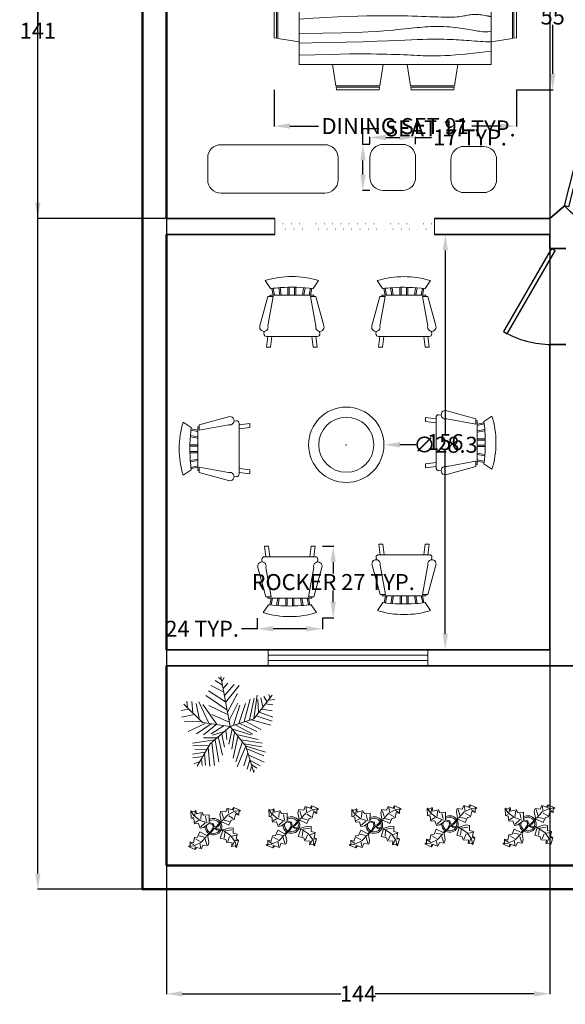
# Model space of a CAD drawing. Units: inches. Extents: x 823 to 1335, y 207 to 1074.
# Tile 1 of 6: x 823 to 1028, y 207 to 577. Entities that reach past the tile are written whole.
import ezdxf

# ---------------------------------------------------------------- set-up
doc = ezdxf.new("R2010")
doc.units = ezdxf.units.IN
doc.header["$MEASUREMENT"] = 0
doc.linetypes.add('ACAD_ISO07W100', pattern=[3, 0, -3])
for name, color, linetype, lineweight in [('A-ANNO-DIMS', 2, 'Continuous', 18), ('A-GLAZ-OVHD', 211, 'ACAD_ISO07W100', 18), ('doors', 51, 'Continuous', 25), ('furniture', 21, 'Continuous', 18), ('inner wall', 102, 'Continuous', 35), ('L-PLNT', 90, 'Continuous', 13), ('outer wall', 105, 'Continuous', 50), ('windows', 211, 'Continuous', 18)]:
    doc.layers.add(name, color=color, linetype=linetype, lineweight=lineweight)
doc.styles.get("Standard").update_dxf_attribs({"font": 'arial.ttf'})
doc.dimstyles.get("Standard").update_dxf_attribs({"dimtxt": 6, "dimasz": 6, "dimexe": 0.18, "dimexo": 0.0625, "dimgap": 0.09, "dimtad": 0, "dimtih": 1, "dimtoh": 1, "dimdec": 0, "dimzin": 0, "dimdsep": 46, "dimlunit": 3, "dimtxsty": 'Standard', "dimcen": 0.09, "dimadec": 0, "dimazin": 0, "dimtfac": 1, "dimtdec": 0, "dimtofl": 0, "dimtmove": 0, "dimatfit": 3, "dimfxl": 1, "dimtolj": 1, "dimtzin": 0, "dimarcsym": 0})

# ---------------------------------------------------------------- blocks, each defined once
blk = doc.blocks.new('*U5')
for p, q in [((0, 0), (0, -6)), ((-40, 0), (-40, -6))]:
    blk.add_line(p, q)
blk.add_lwpolyline([(0, 0), (-34.64, 20), (-35.52, 18.48), (-0.88, -1.52)], close=True)
blk.add_arc((0, 0), 40, 150, 180)
blk = doc.blocks.new('*U4')
for p, q in [((-40, 0), (-40, 6)), ((0, 0), (0, 6))]:
    blk.add_line(p, q)
blk.add_lwpolyline([(0, 0), (-34.64, -20), (-35.52, -18.48), (-0.88, 1.52)], close=True)
blk.add_arc((0, 0), 40, 180, 210)
blk = doc.blocks.new('Dining Set - 36 x 72 in.')
for p, q in [((-22.2343, 26.00059), (-23.4847, 17.99762)), ((-22.2304, 26), (-5.7608, 26)), ((-22, 27.5), (-22.1562, 26.50042)), ((-5.8416, 26.5), (-22.1534, 26.5)), ((-22, 27.5), (-6, 27.5)), ((-5.8437, 26.49966), (-6, 27.5)), ((-4.5152, 17.99762), (-5.7655, 25.99926)), ((5.7657, 26.00059), (4.5153, 17.99762)), ((5.7696, 26), (22.2392, 26)), ((6, 27.5), (5.8438, 26.50042)), ((22.1584, 26.5), (5.8466, 26.5)), ((6, 27.5), (22, 27.5)), ((22.1563, 26.49966), (22, 27.5)), ((23.4848, 17.99762), (22.2345, 25.99926)), ((36, 18), (-36, 18)), ((-36, 18), (-36, -18)), ((36, -18), (36, 18)), ((-45.5, 8), (-44.5004, 8.15617)), ((-45.5, 8), (-45.5, -8)), ((-44.5, -8.15843), (-44.5, 8.15338)), ((-44.0006, 8.23428), (-35.9976, 9.48474)), ((-44, 8.23041), (-44, -8.23915)), ((44.0006, 8.23428), (35.9976, 9.48474)), ((44, 8.23041), (44, -8.23915)), ((44.5, -8.15843), (44.5, 8.15338)), ((45.5, 8), (44.5005, 8.15617)), ((45.5, 8), (45.5, -8)), ((-44.4997, -8.15631), (-45.5, -8)), ((-35.9976, -9.48476), (-43.9993, -8.2345)), ((35.9976, -9.48476), (43.9993, -8.2345)), ((44.4997, -8.15631), (45.5, -8)), ((-36, -18), (36, -18)), ((-22.2343, -26.0006), (-23.4847, -17.99762)), ((-4.5152, -17.99762), (-5.7655, -25.99928)), ((5.7657, -26.0006), (4.5153, -17.99762)), ((23.4848, -17.99762), (22.2345, -25.99928)), ((-22.2304, -26), (-5.7608, -26)), ((-22, -27.5), (-22.1562, -26.50044)), ((-5.8416, -26.5), (-22.1534, -26.5)), ((-22, -27.5), (-6, -27.5)), ((-5.8437, -26.49967), (-6, -27.5)), ((5.7696, -26), (22.2392, -26)), ((6, -27.5), (5.8438, -26.50044)), ((22.1584, -26.5), (5.8466, -26.5)), ((6, -27.5), (22, -27.5)), ((22.1563, -26.49967), (22, -27.5))]:
    blk.add_line(p, q)
for points in [[(-36, 15), (-31.1772, 14.97754), (-26.8079, 14.91406), (-22.8538, 14.81543), (-19.276, 14.6875), (-16.0362, 14.53613), (-13.0957, 14.36718), (-10.4159, 14.18652), (-7.9583, 14), (-5.6904, 13.81315), (-3.6035, 13.63021), (-1.6954, 13.45508), (0.0365, 13.29166), (1.5945, 13.14388), (2.9811, 13.01562), (4.1988, 12.9108), (5.25, 12.83333), (6.1393, 12.78613), (6.8802, 12.76823), (7.4883, 12.77767), (7.9792, 12.8125), (8.3685, 12.87077), (8.6719, 12.95052), (8.9049, 13.0498), (9.0833, 13.16666), (9.2205, 13.29899), (9.3216, 13.44401), (9.3895, 13.59879), (9.4271, 13.76041), (9.4373, 13.92594), (9.4232, 14.09245), (9.3875, 14.257), (9.3333, 14.41666), (9.2638, 14.56917), (9.1836, 14.71484), (9.0975, 14.85465), (9.0104, 14.98958), (8.9272, 15.1206), (8.8529, 15.2487), (8.7922, 15.37483), (8.75, 15.5), (8.7305, 15.62467), (8.7344, 15.74739), (8.7617, 15.86621), (8.8125, 15.97916), (8.8867, 16.08431), (8.9844, 16.17968), (9.1055, 16.26334), (9.25, 16.33333), (9.4189, 16.38802), (9.6172, 16.42708), (9.8506, 16.45052), (10.125, 16.45833), (10.4463, 16.45052), (10.8203, 16.42708), (11.2529, 16.38802), (11.75, 16.33333), (12.3184, 16.26318), (12.9694, 16.17838), (13.7151, 16.07991), (14.5677, 15.96875), (15.5395, 15.84586), (16.6426, 15.71224), (17.8893, 15.56884), (19.2917, 15.41666), (20.859, 15.25667), (22.5879, 15.08984), (24.4721, 14.91715), (26.5052, 14.73958), (28.6809, 14.5581), (30.9929, 14.3737), (33.4347, 14.18733), (36, 14)], [(-36, 10), (-28.9766, 10.14274), (-23.1725, 10.20442), (-18.4241, 10.19775), (-14.5677, 10.13541), (-11.4399, 10.03011), (-8.877, 9.89453), (-6.7154, 9.74137), (-4.7917, 9.58333), (-2.9698, 9.43082), (-1.2246, 9.28515), (0.4415, 9.14534), (2.026, 9.01041), (3.5266, 8.87939), (4.9408, 8.7513), (6.266, 8.62516), (7.5, 8.5), (8.6411, 8.37549), (9.6914, 8.2539), (10.6538, 8.13818), (11.5312, 8.03125), (12.3267, 7.93603), (13.043, 7.85547), (13.6831, 7.79248), (14.25, 7.75), (14.7471, 7.7303), (15.1797, 7.73307), (15.5537, 7.75732), (15.875, 7.80208), (16.1494, 7.86637), (16.3828, 7.94922), (16.5811, 8.04964), (16.75, 8.16666), (16.8944, 8.29915), (17.0143, 8.44531), (17.1089, 8.60319), (17.1771, 8.77083), (17.218, 8.94629), (17.2305, 9.1276), (17.2137, 9.31282), (17.1667, 9.5), (17.0895, 9.6875), (16.987, 9.875), (16.8649, 10.0625), (16.7292, 10.25), (16.5856, 10.4375), (16.4401, 10.625), (16.2985, 10.8125), (16.1667, 11), (16.05, 11.18733), (15.9518, 11.3737), (15.8752, 11.5581), (15.8229, 11.73958), (15.798, 11.91715), (15.8034, 12.08984), (15.842, 12.25667), (15.9167, 12.41666), (16.0295, 12.56836), (16.1784, 12.70833), (16.3605, 12.83268), (16.5729, 12.9375), (16.8127, 13.01888), (17.0768, 13.07291), (17.3625, 13.0957), (17.6667, 13.08333), (17.9894, 13.03312), (18.3418, 12.94726), (18.7382, 12.82918), (19.1927, 12.68229), (19.7195, 12.51001), (20.3327, 12.31575), (21.0465, 12.10294), (21.875, 11.875), (22.8357, 11.63354), (23.959, 11.37304), (25.2786, 11.08618), (26.8282, 10.76562), (28.6414, 10.40405), (30.752, 9.99414), (33.1936, 9.52856), (36, 9)], [(-36, 5.5), (-30.7157, 5.3348), (-26.069, 5.20963), (-21.9946, 5.11767), (-18.4271, 5.05208), (-15.3009, 5.00602), (-12.5508, 4.97265), (-10.1112, 4.94515), (-7.9167, 4.91666), (-5.909, 4.88167), (-4.0586, 4.83984), (-2.3429, 4.79215), (-0.7396, 4.73958), (0.7739, 4.6831), (2.22, 4.6237), (3.6213, 4.56233), (5, 4.5), (6.373, 4.43782), (7.7344, 4.3776), (9.0723, 4.32129), (10.375, 4.27083), (11.6309, 4.22819), (12.8281, 4.19531), (13.9551, 4.17415), (15, 4.16666), (15.954, 4.17448), (16.819, 4.19791), (17.6001, 4.23698), (18.3021, 4.29166), (18.9299, 4.36198), (19.4883, 4.44791), (19.9823, 4.54948), (20.4167, 4.66666), (20.7969, 4.79899), (21.1302, 4.94401), (21.4245, 5.09879), (21.6875, 5.26041), (21.9271, 5.42594), (22.1511, 5.59245), (22.3672, 5.757), (22.5834, 5.91666), (22.8065, 6.06868), (23.0404, 6.21093), (23.2879, 6.34147), (23.5521, 6.45833), (23.8358, 6.55957), (24.142, 6.64323), (24.4735, 6.70735), (24.8334, 6.75), (25.2235, 6.76969), (25.642, 6.76692), (26.0858, 6.74267), (26.5521, 6.69791), (27.0379, 6.63362), (27.5404, 6.55078), (28.0565, 6.45036), (28.5834, 6.33333), (29.1242, 6.19987), (29.7071, 6.04687), (30.3661, 5.87044), (31.1354, 5.66666), (32.0493, 5.43164), (33.142, 5.16146), (34.4475, 4.85221), (36, 4.5)], [(-36, -1), (-30.7915, -0.6591), (-26.0195, -0.38216), (-21.6519, -0.16284), (-17.6563, 0.00521), (-14.0005, 0.12833), (-10.6523, 0.21289), (-7.5796, 0.26522), (-4.75, 0.29166), (-2.134, 0.29793), (0.2878, 0.28711), (2.5317, 0.26163), (4.6146, 0.22396), (6.5529, 0.17651), (8.3633, 0.12174), (10.0623, 0.06209), (11.6667, 0), (13.1899, -0.06201), (14.6341, -0.1211), (15.9982, -0.17432), (17.2813, -0.21875), (18.4823, -0.25147), (19.6003, -0.26953), (20.6343, -0.27002), (21.5834, -0.25), (22.4481, -0.20768), (23.2357, -0.14584), (23.9549, -0.06836), (24.6146, 0.02083), (25.2235, 0.11784), (25.7904, 0.21875), (26.3241, 0.31966), (26.8334, 0.41666), (27.3265, 0.50618), (27.8099, 0.58593), (28.2894, 0.65397), (28.7709, 0.70833), (29.2601, 0.74707), (29.763, 0.76823), (30.2855, 0.76985), (30.8334, 0.75), (31.4088, 0.70784), (31.9994, 0.64713), (32.589, 0.57275), (33.1615, 0.48958), (33.7008, 0.4025), (34.1908, 0.3164), (34.6153, 0.23616), (34.9584, 0.16666), (35.2099, 0.11165), (35.3848, 0.07031), (35.504, 0.04069), (35.5886, 0.02083), (35.6594, 0.00879), (35.7377, 0.0026), (35.8442, 0.00032), (36, 0)], [(-36, -6.5), (-27.1843, -6.31267), (-20.084, -6.1263), (-14.469, -5.9419), (-10.1094, -5.76042), (-6.7752, -5.58285), (-4.2363, -5.41016), (-2.2629, -5.24333), (-0.625, -5.08334), (0.8708, -4.93099), (2.2715, -4.78646), (3.5872, -4.64974), (4.8281, -4.52084), (6.0046, -4.39974), (7.127, -4.28646), (8.2053, -4.18099), (9.25, -4.08334), (10.2705, -3.99382), (11.2734, -3.91407), (12.2647, -3.84603), (13.25, -3.79167), (14.2354, -3.75293), (15.2266, -3.73177), (16.2295, -3.73015), (17.25, -3.75), (18.2912, -3.79248), (19.3451, -3.85547), (20.4009, -3.93604), (21.4479, -4.03125), (22.4754, -4.13819), (23.4727, -4.25391), (24.4289, -4.37549), (25.3334, -4.5), (26.1785, -4.62492), (26.9694, -4.74935), (27.7145, -4.87281), (28.4219, -4.99479), (29.1, -5.11483), (29.7572, -5.23242), (30.4016, -5.34709), (31.0417, -5.45834), (31.6837, -5.56437), (32.3262, -5.65821), (32.9658, -5.73153), (33.599, -5.77604), (34.2224, -5.78345), (34.8327, -5.74545), (35.4264, -5.65373), (36, -5.5)], [(-36, -10), (-26.4022, -9.81299), (-18.4675, -9.62891), (-11.9839, -9.45069), (-6.7396, -9.28125), (-2.5226, -9.12354), (0.8789, -8.98047), (3.6769, -8.85498), (6.0833, -8.75), (8.2767, -8.66765), (10.3021, -8.60677), (12.1712, -8.56543), (13.8958, -8.54167), (15.4876, -8.53353), (16.9583, -8.53907), (18.3197, -8.55632), (19.5834, -8.58334), (20.7616, -8.61841), (21.8685, -8.66081), (22.9188, -8.71004), (23.9271, -8.76563), (24.9081, -8.82707), (25.8763, -8.89388), (26.8465, -8.96558), (27.8334, -9.04167), (28.8474, -9.12118), (29.8828, -9.20117), (30.93, -9.27824), (31.9792, -9.34896), (33.0205, -9.40991), (34.0443, -9.45768), (35.0407, -9.48885), (36, -9.5)], [(-36, -14.5), (-30.0881, -14.33513), (-25.0332, -14.21224), (-20.7312, -14.12647), (-17.0781, -14.07292), (-13.97, -14.04671), (-11.3027, -14.04297), (-8.9724, -14.05681), (-6.875, -14.08334), (-4.9224, -14.11833), (-3.0905, -14.16016), (-1.3709, -14.20785), (0.2448, -14.26042), (1.7647, -14.3169), (3.1973, -14.3763), (4.5507, -14.43767), (5.8333, -14.5), (7.0554, -14.5621), (8.235, -14.62175), (9.3922, -14.67652), (10.5469, -14.72396), (11.7192, -14.76164), (12.929, -14.78711), (14.1965, -14.79794), (15.5417, -14.79167), (16.9933, -14.76424), (18.6152, -14.70508), (20.4804, -14.60197), (22.6615, -14.44271), (25.2312, -14.21509), (28.2624, -13.9069), (31.8277, -13.50594), (36, -13)]]:
    blk.add_lwpolyline(points)
blk = doc.blocks.new('Chair - Rocking')
for p, q in [((-8, -4.5), (-10, -1.5)), ((8, -4.5), (10, -1.5)), ((-8.23428, -6.99939), (-8.3093, -7.47958)), ((-8.23041, -7), (8.23915, -7)), ((-7.5, -4.5), (-7, -7)), ((-6.5, -7), (-7.02225, -4.43)), ((-4.5, -7), (-4.96674, -4.19951)), ((-4, -7), (-4.40532, -4.16272)), ((-1.5, -4.05012), (-1.5, -7)), ((-1, -7), (-1, -4.05012)), ((1, -7), (1, -4.04655)), ((1.5, -4.05012), (1.5, -7)), ((4, -7), (4.40187, -4.18694)), ((4.5, -7), (4.96761, -4.19437)), ((6.5, -7), (7, -4.4057)), ((7.5, -4.5), (7, -7)), ((8.31071, -7.48854), (8.23449, -7.00073)), ((-9, -7.5), (-12, -18.49999)), ((-7, -7.5), (-9, -7.5)), ((-9, -18.49999), (-7, -7.5)), ((7, -7.5), (9, -7.5)), ((9, -18.49999), (7, -7.5)), ((9, -7.5), (12, -18.49999)), ((-10.36644, -20.64523), (-10.5, -21.49999)), ((10.5, -21.49999), (10.3575, -20.58798)), ((-9, -22.49999), (-9.5, -26.49999)), ((0, -22.49999), (-9.5, -22.49999)), ((-8, -26.49999), (-7.5, -22.49999)), ((0, -22.49999), (9.5, -22.49999)), ((8, -26.49999), (7.5, -22.49999)), ((9, -22.49999), (9.5, -26.49999)), ((-9.5, -26.49999), (-8, -26.49999)), ((9.5, -26.49999), (8, -26.49999))]:
    blk.add_line(p, q)
for centre, radius, start, end in [((0, -34.08333), 34.08333, 72.93847, 107.0615), ((0, -68.25004), 64.25, 93.92211, 97.15267), ((0, -68.25004), 64.25, 82.84733, 93.92211), ((-10.5, -18.99999), 1.58114, 161.5651, 18.43495), ((-9.5, -21.49999), 1, 180, 270), ((10.5, -18.99999), 1.58114, 161.5651, 18.43495), ((9.5, -21.49999), 1, 270, 0)]:
    blk.add_arc(centre, radius, start, end)
blk = doc.blocks.new('Plant - Rubber or Philodendron')
for p, q in [((-16.2005, 11.4774), (-13.9899, 8.1064)), ((-16.2005, 11.4774), (-14.8639, 10.7964)), ((-16.0159, 6.3329), (-16.2005, 11.4774)), ((-14.8639, 10.7964), (-12.6195, 11.8975)), ((-13.9899, 8.1064), (-9.5434, 4.7185)), ((-13.3174, 8.325), (-13.0735, 11.0065)), ((-12.6195, 11.8975), (-12.1909, 9.4345)), ((-12.1909, 9.4345), (-8.3829, 10.3)), ((-8.8369, 9.409), (-9.0894, 5.6095)), ((-8.3829, 10.3), (-7.0549, 8.501)), ((-7.0549, 8.501), (-3.0284, 8.6941)), ((-4.8529, 4.012), (-5.7184, 7.82)), ((-3.0284, 8.6941), (-3.0709, 3.1041)), ((4.6914, 8.8812), (5.3859, 11.2828)), ((4.6914, 8.8812), (5.5014, 4.4831)), ((5.3859, 11.2828), (8.8871, 10.7908)), ((5.9878, 10.4842), (7.1971, 6.3869)), ((10.3916, 8.7942), (6.2847, 4.4028)), ((8.8871, 10.7908), (9.9809, 13.4933)), ((9.9809, 13.4933), (13.3837, 12.301)), ((15.3859, 11.3055), (10.3916, 8.7942)), ((10.5828, 12.6946), (10.8893, 9.7953)), ((14.2977, 6.1031), (10.9934, 7.9956)), ((13.3837, 12.301), (14.68, 13.9039)), ((14.5816, 13.2037), (14.3848, 11.8033)), ((14.68, 13.9039), (19.3848, 11.8146)), ((15.7909, 9.1065), (14.8995, 5.3044)), ((15.2875, 10.6053), (17.5907, 9.2105)), ((19.3848, 11.8146), (15.3859, 11.3055)), ((18.1925, 8.4119), (15.7909, 9.1065)), ((19.3848, 11.8146), (18.1868, 10.9119)), ((18.1868, 10.9119), (18.1925, 8.4119)), ((-14.0069, 5.8704), (-16.0159, 6.3329)), ((-15.3434, 6.5514), (-13.9984, 6.9884)), ((-13.5868, 2.2894), (-14.0069, 5.8704)), ((-10.6784, 2.491), (-13.5868, 2.2894)), ((-13.1329, 3.1804), (-10.6614, 4.727)), ((-9.5858, -0.8715), (-10.6784, 2.491)), ((-9.5434, 4.7185), (-4.1917, 2.9888)), ((-9.1318, 0.0195), (-5.9793, 2.9025)), ((-7.1228, -0.443), (-3.5248, 2.2131)), ((-3.5248, 2.2131), (-3.3011, 2.4355)), ((-3.3011, 2.4355), (-0.5306, 1.7947)), ((-3.0709, 3.1041), (0.0797, 2.3163)), ((-0.5306, 1.7947), (-0.2255, -0.5527)), ((-0.5306, 1.7947), (-0.5306, 1.7947)), ((0.0797, 2.3163), (0.4866, -0.031)), ((0.4866, -0.031), (2.1141, 0.2298)), ((2.1141, 0.2298), (5.4346, 3.9146)), ((6.1032, 3.6844), (2.8262, -0.031)), ((5.4346, 3.9146), (5.5014, 4.4831)), ((11.1089, 1.1958), (6.1032, 3.6844)), ((7.7005, 4.8881), (11.5025, 3.9967)), ((12.7005, 4.8994), (11.1089, 1.1958)), ((14.8995, 5.3044), (12.7005, 4.8994)), ((-11.3237, -7.2629), (-9.7321, -3.5593)), ((-6.3237, -7.2516), (-10.1257, -6.3602)), ((-9.7321, -3.5593), (-4.7264, -6.0479)), ((-7.1228, -0.443), (-9.5858, -0.8715)), ((-9.0148, -11.1577), (-4.9047, -6.8122)), ((-2.019, -3.6148), (-4.7264, -6.0479)), ((-4.1246, -6.8466), (-4.0579, -6.2781)), ((-3.3146, -11.2447), (-4.1246, -6.8466)), ((-4.0579, -6.2781), (-0.9375, -3.1608)), ((-2.019, -3.6148), (-0.2255, -0.5527)), ((-0.9375, -3.1608), (0.5883, -0.8135)), ((0.5883, -0.8135), (2.2447, -2.0916)), ((2.8262, -0.031), (1.3003, -0.5527)), ((1.3003, -0.5527), (2.4193, -1.4655)), ((2.2447, -2.0916), (6.7108, -2.6626)), ((2.4193, -1.4655), (6.895, -2.1175)), ((4.943, -7.9659), (6.7108, -2.6626)), ((11.6605, -0.5413), (6.895, -2.1175)), ((12.3677, -6.1981), (7.219, -2.6772)), ((8.125, -4.0768), (7.7715, -7.9659)), ((8.3544, -2.7453), (13.1973, -2.1704)), ((10.2463, -10.4408), (11.6605, -6.9053)), ((11.6605, -0.5413), (14.1354, -0.8948)), ((15.5496, -10.7943), (12.3677, -6.1981)), ((16.2567, -5.8446), (13.4283, -6.5517)), ((14.1354, -0.8948), (14.1354, -4.4304)), ((14.1354, -4.4304), (16.9638, -5.1375)), ((16.9638, -5.1375), (16.2567, -8.673)), ((-18.008, -14.1781), (-16.8101, -13.2754)), ((-18.008, -14.1781), (-14.0091, -13.669)), ((-16.8157, -10.7754), (-14.4141, -11.4699)), ((-16.8101, -13.2754), (-16.8157, -10.7754)), ((-13.9107, -12.9688), (-16.2139, -11.574)), ((-14.4141, -11.4699), (-13.5228, -7.6679)), ((-14.0091, -13.669), (-9.0148, -11.1577)), ((-13.5228, -7.6679), (-11.3237, -7.2629)), ((-12.921, -8.4665), (-9.6166, -10.359)), ((-9.206, -15.0581), (-9.5126, -12.1588)), ((-7.5103, -13.1543), (-8.6042, -15.8568)), ((-4.0092, -13.6463), (-7.5103, -13.1543)), ((-4.611, -12.8477), (-5.8203, -8.7504)), ((-3.3146, -11.2447), (-4.0092, -13.6463)), ((8.8321, -9.0266), (4.943, -7.9659)), ((9.5392, -11.1479), (8.8321, -9.0266)), ((13.4283, -11.5015), (9.5392, -11.1479)), ((13.0748, -13.9763), (13.4283, -11.5015)), ((15.5496, -13.6228), (13.0748, -13.9763)), ((14.8425, -10.7943), (13.7819, -13.2692)), ((16.6103, -14.6834), (15.5496, -10.7943)), ((16.6103, -14.6834), (15.5496, -13.6228)), ((17.3174, -9.7337), (15.9032, -9.7337)), ((16.2567, -8.673), (18.0245, -9.7337)), ((18.0245, -9.7337), (16.6103, -14.6834)), ((-13.3032, -16.2674), (-18.008, -14.1781)), ((-12.0069, -14.6645), (-13.3032, -16.2674)), ((-13.2048, -15.5672), (-13.008, -14.1668)), ((-8.6042, -15.8568), (-12.0069, -14.6645))]:
    blk.add_line(p, q)
for centre, radius, start, end in [((0.0308, 0.1664), 6, 178.6147, 235.1169), ((0.0308, 0.1664), 5, 168.1647, 238.6725), ((0, 0), 6.1275, 34.37569, 120.1028), ((-0.0601, -0.2075), 5.2461, 33.82192, 124.9414), ((-0.2664, 0.1682), 5.2775, 338.4094, 20.03007), ((-0.098, 0.1364), 6.1288, 341.2017, 26.09184), ((-0.0234, 0.3825), 6.1492, 242.5812, 331.2714), ((-0.1102, 0.4886), 5.2883, 247.3711, 327.472)]:
    blk.add_arc(centre, radius, start, end)
blk = doc.blocks.new('*U20')
for p, q in [((0, 0), (-10.5, 57)), ((-7.288, 39.707), (-21.778, 46.673)), ((-8.737, 47.138), (-17.069, 52.711)), ((-10.186, 53.64), (-13.084, 55.962)), ((-9.099, 51.782), (-6.563, 55.962)), ((-7.65, 43.423), (-2.578, 49.46)), ((-5.839, 35.992), (4.667, 48.067)), ((-5.114, 27.632), (10.463, 46.673)), ((-3.665, 19.273), (-27.574, 35.527)), ((-5.114, 28.097), (-24.676, 40.636)), ((-2.941, 16.486), (8.652, 37.85)), ((27, 9), (48, 36)), ((27.127, 9.056), (31.112, 35.992)), ((38.719, 34.134), (41.979, 28.561)), ((44.153, 36.456), (45.239, 32.741)), ((-31.5, 4.5), (-52.5, 25.5)), ((-48.585, 21.131), (-49.309, 29.026)), ((-43.513, 28.561), (-42.427, 15.558)), ((-38.442, 26.239), (-34.819, 7.663)), ((-35.544, 28.097), (-24.314, 3.947)), ((-14.533, 2.09), (-30.834, 25.31)), ((-24.314, 23.917), (-2.941, 13.7)), ((-1.129, 6.734), (9.014, 26.704)), ((3.942, 1.625), (11.187, 24.381)), ((10.101, 3.483), (17.708, 26.239)), ((16.259, 5.805), (23.142, 31.348)), ((22.055, 7.198), (27.489, 32.277)), ((31.836, 30.883), (32.561, 16.486)), ((35.096, 32.741), (37.27, 22.524)), ((40.53, 25.775), (48.862, 24.846)), ((43.791, 29.954), (51.036, 30.883)), ((-47.498, 19.737), (-55.83, 18.344)), ((-40.615, 13.7), (-55.105, 10.913)), ((-20.691, 13.7), (-1.129, 4.876)), ((29.662, 12.307), (48.137, 6.269)), ((33.285, 16.486), (48.862, 10.913)), ((36.183, 19.737), (48.137, 17.88)), ((-33.37, 6.269), (-52.207, 5.34)), ((-28.299, 3.483), (-47.86, -5.805)), ((-21.416, 3.018), (-38.079, -8.128)), ((0, 0), (-31.5, 4.5)), ((-15.982, 2.09), (-30.11, -9.521)), ((0, 0), (-22.5, -19.5)), ((-6.563, 1.161), (-21.416, -8.128)), ((0, 0), (27, 9)), ((0, 0), (18, -22.5)), ((6.478, 1.625), (26.04, -8.592)), ((11.187, 3.483), (30.749, -5.805)), ((18.07, 5.805), (35.096, -3.483)), ((24.229, 7.663), (46.688, 1.625)), ((-6.563, -5.805), (-19.967, -9.985)), ((-9.461, -8.592), (-6.201, -23.453)), ((-4.752, -3.483), (-3.665, -14.629)), ((2.493, -3.019), (-1.491, -20.202)), ((1.769, -2.555), (24.229, -9.521)), ((5.029, -6.27), (2.131, -25.775)), ((7.565, -9.056), (32.198, -14.629)), ((-17.431, -15.094), (-42.789, -18.809)), ((-24.314, -21.596), (-42.427, -22.06)), ((-22.5, -19.5), (-37.5, -45)), ((-15.257, -12.772), (-30.11, -12.772)), ((-20.691, -18.345), (-17.793, -44.352)), ((-17.069, -15.094), (-12.721, -40.172)), ((-13.446, -11.378), (-8.737, -32.741)), ((9.014, -11.378), (3.58, -35.992)), ((14.085, -16.951), (6.478, -40.172)), ((12.274, -15.094), (36.907, -18.809)), ((16.259, -19.738), (36.183, -22.989)), ((-28.299, -29.026), (-42.789, -31.348)), ((-26.849, -26.24), (-40.253, -25.775)), ((-29.023, -30.884), (-27.936, -43.887)), ((-25.038, -23.918), (-22.865, -45.281)), ((18.07, -22.524), (8.289, -45.745)), ((20.244, -30.419), (15.897, -44.816)), ((18, -22.5), (27, -52.5)), ((18.433, -22.524), (40.53, -29.026)), ((19.157, -25.311), (38.719, -33.206)), ((21.331, -32.741), (39.081, -40.636)), ((-30.834, -34.135), (-42.427, -35.528)), ((-34.457, -39.708), (-40.978, -42.494)), ((-32.646, -36.921), (-31.921, -44.352)), ((22.78, -37.85), (19.519, -48.532)), ((22.78, -38.314), (34.372, -44.816)), ((24.591, -43.423), (30.749, -47.603)), ((24.591, -45.745), (23.142, -50.854)), ((26.764, -49.925), (28.213, -50.854))]:
    blk.add_line(p, q)
blk = doc.blocks.new('WIN-60IN')
for p, q in [((0, 0), (0, 60)), ((0, 60), (6, 60)), ((2, 0), (2, 60)), ((4, 60), (4, 0)), ((6, 60), (6, 0)), ((6, 0), (0, 0))]:
    blk.add_line(p, q)
blk = doc.blocks.new('SEAT-HALL-SINGLE')
for points in [[(5, 17.36), (12.18, 17.36)], [(0, 5), (0, 12.36)], [(17.18, 12.36), (17.18, 5)], [(12.18, 0), (5, 0)]]:
    blk.add_lwpolyline(points)
for centre, start, end in [((5, 12.36), 90, 180), ((12.18, 12.36), 0, 90), ((5, 5), 180, 270), ((12.18, 5), 270, 0)]:
    blk.add_arc(centre, 5, start, end)
blk = doc.blocks.new('*D30')
at = {"layer": 'A-ANNO-DIMS', "color": 0, "lineweight": -2, "transparency": 16777216}
for p, q in [((918.69, 550.91), (918.69, 537.15)), ((1009.69, 550.91), (1009.69, 537.15)), ((924.69, 537.33), (935.39, 537.33)), ((1003.69, 537.33), (993, 537.33))]:
    blk.add_line(p, q, dxfattribs=at)
for points in [[(924.69, 538.33), (924.69, 536.33), (918.69, 537.33)], [(1003.69, 538.33), (1003.69, 536.33), (1009.69, 537.33)]]:
    blk.add_solid(points, dxfattribs=at)
at = {"layer": 'Defpoints', "color": 0, "lineweight": -2, "transparency": 16777216}
for p in [(918.69, 550.98), (1009.69, 550.98), (1009.69, 537.33)]:
    blk.add_point(p, dxfattribs=at)
at = {"layer": 'A-ANNO-DIMS', "color": 0, "transparency": 16777216, "insert": (964.19, 537.33), "char_height": 6, "attachment_point": 5}
blk.add_mtext('\\A1;DINING SET 91', dxfattribs=at)
blk = doc.blocks.new('*D31')
at = {"layer": 'A-ANNO-DIMS', "color": 0, "lineweight": -2, "transparency": 16777216}
for p, q in [((1009.76, 605.98), (1023.52, 605.98)), ((1023.34, 599.98), (1023.34, 581.62)), ((1023.34, 556.98), (1023.34, 575.34)), ((1009.76, 550.98), (1023.52, 550.98))]:
    blk.add_line(p, q, dxfattribs=at)
for points in [[(1022.34, 599.98), (1024.34, 599.98), (1023.34, 605.98)], [(1022.34, 556.98), (1024.34, 556.98), (1023.34, 550.98)]]:
    blk.add_solid(points, dxfattribs=at)
at = {"layer": 'Defpoints', "color": 0, "lineweight": -2, "transparency": 16777216}
for p in [(1009.69, 605.98), (1023.34, 605.98), (1009.69, 550.98)]:
    blk.add_point(p, dxfattribs=at)
at = {"layer": 'A-ANNO-DIMS', "color": 0, "transparency": 16777216, "insert": (1023.34, 578.48), "char_height": 6, "attachment_point": 5}
blk.add_mtext('\\A1;55', dxfattribs=at)
blk = doc.blocks.new('*D34')
at = {"layer": 'A-ANNO-DIMS', "color": 0, "lineweight": -2, "transparency": 16777216}
for p, q in [((936.93, 379.54), (941.1, 379.54)), ((940.92, 373.54), (940.92, 369.24)), ((940.92, 358.54), (940.92, 362.85)), ((936.93, 352.54), (941.1, 352.54))]:
    blk.add_line(p, q, dxfattribs=at)
for points in [[(939.92, 373.54), (941.92, 373.54), (940.92, 379.54)], [(939.92, 358.54), (941.92, 358.54), (940.92, 352.54)]]:
    blk.add_solid(points, dxfattribs=at)
at = {"layer": 'Defpoints', "color": 0, "lineweight": -2, "transparency": 16777216}
for p in [(936.87, 379.54), (936.87, 352.54), (940.92, 352.54)]:
    blk.add_point(p, dxfattribs=at)
at = {"layer": 'A-ANNO-DIMS', "color": 0, "transparency": 16777216, "insert": (940.92, 366.04), "char_height": 6, "attachment_point": 5}
blk.add_mtext('\\A1;ROCKER 27 TYP.', dxfattribs=at)
blk = doc.blocks.new('*D35')
at = {"layer": 'A-ANNO-DIMS', "color": 0, "lineweight": -2, "transparency": 16777216}
for p, q in [((912.43, 352.48), (912.43, 348.31)), ((936.87, 352.48), (936.87, 348.31)), ((912.43, 348.49), (906.43, 348.49)), ((930.87, 348.49), (918.43, 348.49))]:
    blk.add_line(p, q, dxfattribs=at)
for points in [[(918.43, 349.49), (918.43, 347.49), (912.43, 348.49)], [(930.87, 349.49), (930.87, 347.49), (936.87, 348.49)]]:
    blk.add_solid(points, dxfattribs=at)
at = {"layer": 'Defpoints', "color": 0, "lineweight": -2, "transparency": 16777216}
for p in [(912.43, 352.54), (936.87, 352.54), (912.43, 348.49)]:
    blk.add_point(p, dxfattribs=at)
at = {"layer": 'A-ANNO-DIMS', "color": 0, "transparency": 16777216, "insert": (891.69, 348.49), "char_height": 6, "attachment_point": 5}
blk.add_mtext('\\A1;24 TYP.', dxfattribs=at)
blk = doc.blocks.new('*D38')
at = {"layer": 'A-ANNO-DIMS', "color": 0, "lineweight": -2, "transparency": 16777216}
for p, q in [((952.1, 530.45), (952.1, 536.45)), ((952.1, 536.45), (958.1, 536.45)), ((954.64, 530.45), (951.92, 530.45)), ((952.1, 519.09), (952.1, 524.45)), ((954.64, 513.09), (951.92, 513.09))]:
    blk.add_line(p, q, dxfattribs=at)
for points in [[(951.1, 524.45), (953.1, 524.45), (952.1, 530.45)], [(951.1, 519.09), (953.1, 519.09), (952.1, 513.09)]]:
    blk.add_solid(points, dxfattribs=at)
at = {"layer": 'Defpoints', "color": 0, "lineweight": -2, "transparency": 16777216}
for p in [(952.1, 530.45), (954.7, 530.45), (954.7, 513.09)]:
    blk.add_point(p, dxfattribs=at)
at = {"layer": 'A-ANNO-DIMS', "color": 0, "transparency": 16777216, "insert": (984.89, 536.45), "char_height": 6, "attachment_point": 5}
blk.add_mtext('\\A1;SEAT 17 TYP.', dxfattribs=at)
blk = doc.blocks.new('*D39')
at = {"layer": 'A-ANNO-DIMS', "color": 0, "lineweight": -2, "transparency": 16777216}
for p, q in [((954.7, 530.51), (954.7, 533.23)), ((960.7, 533.05), (965.88, 533.05)), ((971.88, 530.51), (971.88, 533.23)), ((971.88, 533.05), (977.88, 533.05))]:
    blk.add_line(p, q, dxfattribs=at)
for points in [[(960.7, 534.05), (960.7, 532.05), (954.7, 533.05)], [(965.88, 534.05), (965.88, 532.05), (971.88, 533.05)]]:
    blk.add_solid(points, dxfattribs=at)
at = {"layer": 'Defpoints', "color": 0, "lineweight": -2, "transparency": 16777216}
for p in [(971.88, 533.05), (954.7, 530.45), (971.88, 530.45)]:
    blk.add_point(p, dxfattribs=at)
at = {"layer": 'A-ANNO-DIMS', "color": 0, "transparency": 16777216, "insert": (992.3, 533.05), "char_height": 6, "attachment_point": 5}
blk.add_mtext('\\A1;17 TYP.', dxfattribs=at)
blk = doc.blocks.new('*D57')
at = {"layer": 'A-ANNO-DIMS', "color": 0, "lineweight": -2, "transparency": 16777216}
for p, q in [((869.2, 1030.61), (829.83, 1030.61)), ((830.01, 1024.61), (830.01, 643.76)), ((830.01, 256.61), (830.01, 637.45)), ((869.2, 250.61), (829.83, 250.61))]:
    blk.add_line(p, q, dxfattribs=at)
for points in [[(829.01, 1024.61), (831.01, 1024.61), (830.01, 1030.61)], [(829.01, 256.61), (831.01, 256.61), (830.01, 250.61)]]:
    blk.add_solid(points, dxfattribs=at)
at = {"layer": 'Defpoints', "color": 0, "lineweight": -2, "transparency": 16777216}
for p in [(830.01, 1030.61), (869.26, 1030.61), (869.26, 250.61)]:
    blk.add_point(p, dxfattribs=at)
at = {"layer": 'A-ANNO-DIMS', "color": 0, "transparency": 16777216, "insert": (830.01, 640.61), "char_height": 6, "attachment_point": 5}
blk.add_mtext('\\A1;780', dxfattribs=at)
blk = doc.blocks.new('*D60')
at = {"layer": 'A-ANNO-DIMS', "color": 0, "lineweight": -2, "transparency": 16777216}
for p, q in [((878.26, 775.54), (878.26, 211.18)), ((1022.26, 775.54), (1022.26, 211.18)), ((884.26, 211.36), (943.84, 211.36)), ((1016.26, 211.36), (956.69, 211.36))]:
    blk.add_line(p, q, dxfattribs=at)
for points in [[(884.26, 212.36), (884.26, 210.36), (878.26, 211.36)], [(1016.26, 212.36), (1016.26, 210.36), (1022.26, 211.36)]]:
    blk.add_solid(points, dxfattribs=at)
at = {"layer": 'Defpoints', "color": 0, "lineweight": -2, "transparency": 16777216}
for p in [(878.26, 775.61), (1022.26, 775.61), (1022.26, 211.36)]:
    blk.add_point(p, dxfattribs=at)
at = {"layer": 'A-ANNO-DIMS', "color": 0, "transparency": 16777216, "insert": (950.26, 211.36), "char_height": 6, "attachment_point": 5}
blk.add_mtext('\\A1;144', dxfattribs=at)
blk = doc.blocks.new('*D67')
at = {"layer": 'A-ANNO-DIMS', "color": 0, "lineweight": -2, "transparency": 16777216}
for p, q in [((878.2, 643.61), (829.83, 643.61)), ((830.01, 637.61), (830.01, 576.21)), ((830.01, 508.61), (830.01, 570)), ((878.2, 502.61), (829.83, 502.61))]:
    blk.add_line(p, q, dxfattribs=at)
for points in [[(829.01, 637.61), (831.01, 637.61), (830.01, 643.61)], [(829.01, 508.61), (831.01, 508.61), (830.01, 502.61)]]:
    blk.add_solid(points, dxfattribs=at)
at = {"layer": 'Defpoints', "color": 0, "lineweight": -2, "transparency": 16777216}
for p in [(878.26, 643.61), (830.01, 502.61), (878.26, 502.61)]:
    blk.add_point(p, dxfattribs=at)
at = {"layer": 'A-ANNO-DIMS', "color": 0, "transparency": 16777216, "insert": (830.01, 573.11), "char_height": 6, "attachment_point": 5}
blk.add_mtext('\\A1;141', dxfattribs=at)
blk = doc.blocks.new('*D73')
at = {"layer": 'A-ANNO-DIMS', "color": 0, "lineweight": -2, "transparency": 16777216}
for p, q in [((878.26, 340.54), (878.26, 211.18)), ((1022.26, 340.54), (1022.26, 211.18)), ((884.26, 211.36), (943.84, 211.36)), ((1016.26, 211.36), (956.69, 211.36))]:
    blk.add_line(p, q, dxfattribs=at)
for points in [[(884.26, 212.36), (884.26, 210.36), (878.26, 211.36)], [(1016.26, 212.36), (1016.26, 210.36), (1022.26, 211.36)]]:
    blk.add_solid(points, dxfattribs=at)
at = {"layer": 'Defpoints', "color": 0, "lineweight": -2, "transparency": 16777216}
for p in [(878.26, 340.61), (1022.26, 340.61), (1022.26, 211.36)]:
    blk.add_point(p, dxfattribs=at)
at = {"layer": 'A-ANNO-DIMS', "color": 0, "transparency": 16777216, "insert": (950.26, 211.36), "char_height": 6, "attachment_point": 5}
blk.add_mtext('\\A1;144', dxfattribs=at)
blk = doc.blocks.new('*D74')
at = {"layer": 'A-ANNO-DIMS', "color": 0, "lineweight": -2, "transparency": 16777216}
for p, q in [((1022.2, 496.61), (982.83, 496.61)), ((983.01, 490.61), (983.01, 421.76)), ((983.01, 346.61), (983.01, 415.45)), ((1022.2, 340.61), (982.83, 340.61))]:
    blk.add_line(p, q, dxfattribs=at)
for points in [[(982.01, 490.61), (984.01, 490.61), (983.01, 496.61)], [(982.01, 346.61), (984.01, 346.61), (983.01, 340.61)]]:
    blk.add_solid(points, dxfattribs=at)
at = {"layer": 'Defpoints', "color": 0, "lineweight": -2, "transparency": 16777216}
for p in [(983.01, 496.61), (1022.26, 496.61), (1022.26, 340.61)]:
    blk.add_point(p, dxfattribs=at)
at = {"layer": 'A-ANNO-DIMS', "color": 0, "transparency": 16777216, "insert": (983.01, 418.61), "char_height": 6, "attachment_point": 5}
blk.add_mtext('\\A1;156', dxfattribs=at)
blk = doc.blocks.new('*D84')
at = {"layer": 'A-ANNO-DIMS', "color": 0, "lineweight": -2, "transparency": 16777216}
for p, q in [((945.74, 417.61), (945.92, 417.61)), ((945.83, 417.52), (945.83, 417.7)), ((971.98, 417.61), (965.98, 417.61))]:
    blk.add_line(p, q, dxfattribs=at)
blk.add_solid([(965.98, 418.61), (965.98, 416.61), (959.98, 417.61)], dxfattribs=at)
at = {"layer": 'Defpoints', "color": 0, "lineweight": -2, "transparency": 16777216}
for p in [(931.68, 417.61), (959.98, 417.61)]:
    blk.add_point(p, dxfattribs=at)
at = {"layer": 'A-ANNO-DIMS', "color": 0, "transparency": 16777216, "insert": (983.12, 417.61), "char_height": 6, "attachment_point": 5}
blk.add_mtext('\\A1;∅28.3', dxfattribs=at)

msp = doc.modelspace()

# ---------------------------------------------------------------- linework, layer by layer
at = {"layer": 'A-GLAZ-OVHD'}
for p, q in [((918.95, 500.61), (978.95, 500.61)), ((978.95, 498.61), (918.95, 498.61))]:
    msp.add_line(p, q, dxfattribs=at)
at = {"layer": 'furniture'}
for p, q in [((898.8, 530.34), (937.77, 530.34)), ((893.8, 517.12), (893.8, 525.34)), ((942.77, 525.34), (942.77, 517.12)), ((937.77, 512.12), (898.8, 512.12))]:
    msp.add_line(p, q, dxfattribs=at)
for radius in [14.15, 10.35]:
    msp.add_circle((945.83, 417.61), radius, dxfattribs=at)
for centre, start, end in [((898.8, 525.34), 90, 180), ((937.77, 525.34), 0, 90), ((898.8, 517.12), 180, 270), ((937.77, 517.12), 270, 0)]:
    msp.add_arc(centre, 5, start, end, dxfattribs=at)
at = {"layer": 'inner wall'}
for p, q in [((1022.26, 502.61), (1027.79, 507.38)), ((1027.79, 507.38), (1033.71, 501.63)), ((918.95, 502.61), (878.26, 502.61)), ((1022.26, 502.61), (978.95, 502.61)), ((918.95, 496.61), (878.26, 496.61)), ((1022.26, 496.61), (978.95, 496.61)), ((1022.26, 491.3), (1022.26, 496.61)), ((1022.26, 491.3), (1022.26, 496.61)), ((1022.26, 340.61), (1022.26, 455.3)), ((1022.26, 340.61), (1022.26, 455.3)), ((1022.26, 340.61), (878.26, 340.61)), ((1088.26, 334.61), (878.26, 334.61))]:
    msp.add_line(p, q, dxfattribs=at)
for points in [[(1028.26, 491.3), (1022.26, 491.3)], [(1022.26, 455.3), (1028.26, 455.3)]]:
    msp.add_lwpolyline(points, dxfattribs=at)
at = {"layer": 'outer wall'}
for p, q in [((878.26, 502.61), (878.26, 643.61)), ((878.26, 340.61), (878.26, 496.61)), ((878.26, 259.61), (878.26, 334.61)), ((1280.26, 259.61), (878.26, 259.61))]:
    msp.add_line(p, q, dxfattribs=at)
msp.add_lwpolyline([(869.26, 1030.61), (1289.26, 1030.61), (1289.26, 250.61), (869.26, 250.61)], close=True, dxfattribs=at)
at = {"layer": 'windows'}
for p, q in [((918.95, 496.61), (918.95, 502.61)), ((978.95, 502.61), (978.95, 496.61))]:
    msp.add_line(p, q, dxfattribs=at)

# ---------------------------------------------------------------- block references
at = {"layer": 'doors'}
for name, p, xscale, yscale, zscale, rotation in [('*U4', (1027.79, 507.38), 0.9000000000000001, 0.9000000000000001, 0.9000000000000001, 225.7621076971286), ('*U5', (1022.86, 491.3), 0.9, 0.9, 0.9, 90)]:
    msp.add_blockref(name, p, dxfattribs=dict(at, xscale=xscale, yscale=yscale, zscale=zscale, rotation=rotation))
at = {"layer": 'furniture'}
for name, p in [('Dining Set - 36 x 72 in.', (964.19, 578.48)), ('SEAT-HALL-SINGLE', (954.7, 513.09)), ('Chair - Rocking', (925.42, 480.79)), ('Chair - Rocking', (967.46, 480.77))]:
    msp.add_blockref(name, p, dxfattribs=at)
for name, p, rotation in [('SEAT-HALL-SINGLE', (1002.29, 529.69), 180), ('Chair - Rocking', (1002.03, 418.4), 270), ('Chair - Rocking', (883.11, 416.14), 90), ('Chair - Rocking', (924.65, 353.04), 180), ('Chair - Rocking', (967.51, 353.82), 180)]:
    msp.add_blockref(name, p, dxfattribs=dict(at, rotation=rotation))
at = {"layer": 'L-PLNT'}
for name, p, xscale, yscale, zscale in [('*U20', (902.17, 311.75), 0.3294393859005505, 0.3294393859005505, 0.3294393859005505), ('Plant - Rubber or Philodendron', (895.94, 274.05), 0.5226467583176748, 0.5226467583176748, 0.5226467583176748), ('Plant - Rubber or Philodendron', (925.22, 274.66), 0.5226467583176748, 0.5226467583176748, 0.5226467583176748), ('Plant - Rubber or Philodendron', (956.34, 274.66), 0.5226467583176748, 0.5226467583176748, 0.5226467583176748), ('Plant - Rubber or Philodendron', (984.71, 275.07), 0.5226467583176748, 0.5226467583176748, 0.5226467583176748), ('Plant - Rubber or Philodendron', (1013.99, 275.07), 0.5226467583176748, 0.5226467583176748, 0.5226467583176748)]:
    msp.add_blockref(name, p, dxfattribs=dict(at, xscale=xscale, yscale=yscale, zscale=zscale))
at = {"layer": 'windows', "rotation": 270.0000000000002}
msp.add_blockref('WIN-60IN', (916.47, 340.61), dxfattribs=at)

# ---------------------------------------------------------------- dimensions: what is measured, and where the dimension line sits
at = {"layer": 'A-ANNO-DIMS'}
for base, p1, p2, picture, middle in [((830.01, 1030.61), (869.26, 250.61), (869.26, 1030.61), '*D57', (830.01, 640.61)), ((830.01, 502.61), (878.26, 643.61), (878.26, 502.61), '*D67', (830.01, 573.11)), ((1023.34, 605.98), (1009.69, 550.98), (1009.69, 605.98), '*D31', (1023.34, 578.48)), ((983.01, 496.61), (1022.26, 340.61), (1022.26, 496.61), '*D74', (983.01, 418.61))]:
    dim = msp.add_linear_dim(base=base, p1=p1, p2=p2, angle=90, dimstyle='Standard', override={"dimdec": 0, "dimlfac": 1, "dimrnd": 0, "dimzin": 0, "dimdsep": 46, "dimlunit": 2}, dxfattribs=at)
    dim.commit()
    dim.dimension.update_dxf_attribs({"geometry": picture, "text_midpoint": middle})
for p1, p2, picture in [((878.26, 775.61), (1022.26, 775.61), '*D60'), ((878.26, 340.61), (1022.26, 340.61), '*D73')]:
    dim = msp.add_linear_dim(base=(1022.26, 211.36), p1=p1, p2=p2, dimstyle='Standard', override={"dimdec": 0, "dimlfac": 1, "dimrnd": 0, "dimzin": 0, "dimdsep": 46, "dimlunit": 2}, dxfattribs=at)
    dim.commit()
    dim.dimension.update_dxf_attribs({"geometry": picture, "text_midpoint": (950.26, 211.36)})
for base, p1, p2, text, picture, middle in [((1009.69, 537.33), (918.69, 550.98), (1009.69, 550.98), 'DINING SET <>', '*D30', (964.19, 537.33)), ((971.88, 533.05), (954.7, 530.45), (971.88, 530.45), '<> TYP.', '*D39', (992.3, 533.05))]:
    dim = msp.add_linear_dim(base=base, p1=p1, p2=p2, text=text, dimstyle='Standard', override={"dimdec": 0, "dimlfac": 1, "dimrnd": 0, "dimzin": 0, "dimdsep": 46, "dimlunit": 2}, dxfattribs=at)
    dim.commit()
    dim.dimension.update_dxf_attribs({"geometry": picture, "text_midpoint": middle})
for base, p1, p2, angle, text, picture, middle in [((952.1, 530.45), (954.7, 513.09), (954.7, 530.45), 90, 'SEAT <> TYP.', '*D38', (984.89, 536.45)), ((940.92, 352.54), (936.87, 379.54), (936.87, 352.54), 270, 'ROCKER <> TYP.', '*D34', (940.92, 366.04)), ((912.43, 348.49), (936.87, 352.54), (912.43, 352.54), 180, '<> TYP.', '*D35', (891.69, 348.49))]:
    dim = msp.add_linear_dim(base=base, p1=p1, p2=p2, angle=angle, text=text, dimstyle='Standard', override={"dimdec": 0, "dimlfac": 1, "dimrnd": 0, "dimzin": 0, "dimdsep": 46, "dimlunit": 2}, dxfattribs=at)
    dim.commit()
    dim.dimension.update_dxf_attribs({"geometry": picture, "text_midpoint": middle})
dim = msp.add_diameter_dim_2p(p1=(931.68, 417.61), p2=(959.98, 417.61), dimstyle='Standard', override={"dimdec": 1, "dimlfac": 1, "dimrnd": 0, "dimzin": 0, "dimdsep": 46, "dimlunit": 2}, dxfattribs=at)
dim.commit()
dim.dimension.update_dxf_attribs({"geometry": '*D84', "text_midpoint": (971.98, 417.61), "dimtype": 163})

doc.saveas('drawing.dxf')
